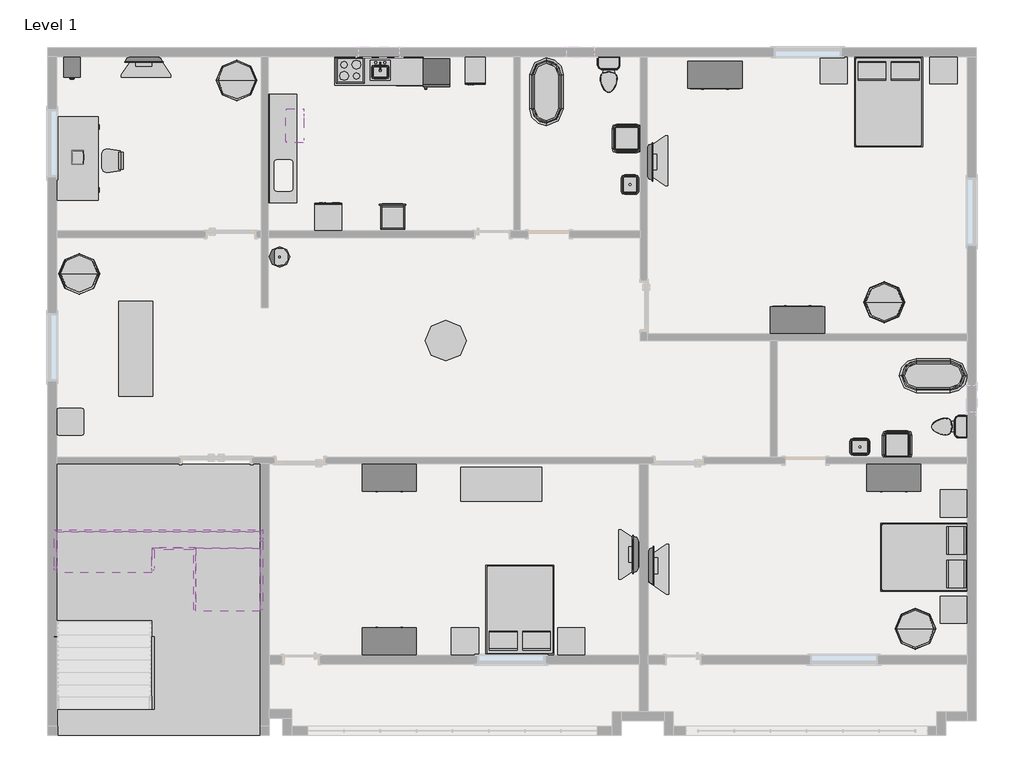
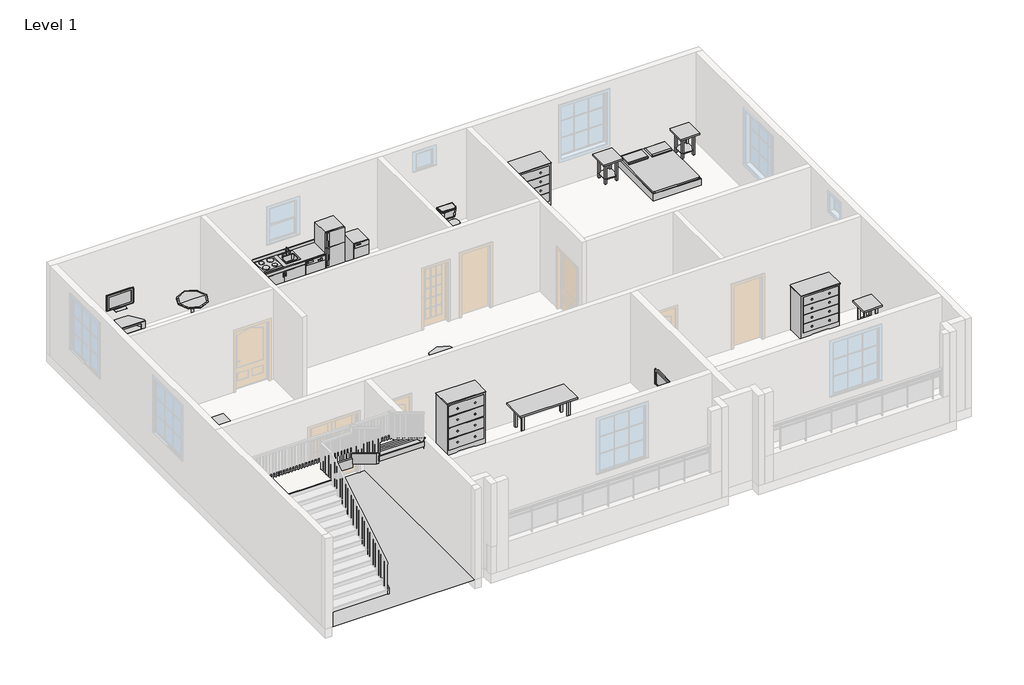
# One storey, part 4 of 4: 35 furniture elements, 10 proxies, 9 members, 8 flow terminals, 2 geographic elements, 1 slab, 1 stair flight.
"""IFC4 building model written with IfcOpenShell, lengths in millimetres."""

from ifc_helpers import new_model, si_unit, frame, origin, place, context, project, spatial, polyline, outline, extrude, faceted_brep, triangles, transform, mapped, element, save
from components import entourage_4c8cfd20, proxy_7e1014cc, proxy_a6faaae8, proxy_45b28599, kitchenette_medium_kitchenette_medium_844211aa, proxy_8a8d5ab2, proxy_8b8c2dc4, proxy_c523a7b7, flow_terminal_871c2e40, flow_terminal_d49f872f, flow_terminal_62a433f7, toilet_domestic_3d_toilet_domestic_3d_f7549cf7, toilet_domestic_3d_toilet_domestic_3d_183bbd19, flow_terminal_b374fae2, furniture_1d2926bd, furniture_d4d3357e, chair_desk_chair_desk_ccc35c8f, furniture_22cae41e, furniture_c6510c7c, furniture_2fc54265, furniture_2babcf72, furniture_9fa109b2, furniture_56245f3a, tv_stand_tv_stand_6ce107e5, furniture_92191dda, furniture_905aceb5, furniture_bcf351fa, furniture_5bc9ed15, furniture_a5b052b6, furniture_c80d6d9c, trash_can_trash_can_952d1acd, non_monolithic_landing_e2aaf49c, stair_flight_724757b1

model = new_model("IFC4")

# Units and contexts
model_context = context("Model", 3, world=origin())
ifc_project = project(units=[si_unit("LENGTHUNIT", "METRE", prefix="MILLI")], contexts=[model_context])

# Site, building, storey
site = spatial("IfcSite", under=ifc_project)
building = spatial("IfcBuilding", under=site)
storey = spatial("IfcBuildingStorey", under=building, Name="Level 1", Elevation=0.0)

# Proxies
placement = place(None, origin())
element("IfcBuildingElementProxy", 1, Name="Building Element Proxy", at=placement, inside=storey, context=model_context, shape_type="Tessellation", body=[
    triangles([(-19977.248053, 5318.025975, 0.0), (-15405.248053, 5318.025975, 0.0), (-15405.248053, -777.9740976, 0.0), (-19951.8472778, -777.9740976, 0.0)], [[1, 4, 2], [3, 2, 4]], closed=False),
])
entourage_shape = entourage_4c8cfd20(model_context)
element("IfcBuildingElementProxy", 2, Name="Entourage", at=placement, inside=storey, context=model_context, shape_type="MappedRepresentation", body=[
    mapped(entourage_shape, transform((-19545.4480019, 12201.4258877, 762.0), x_axis=(0.0, 1.0000000000000002, 0.0), y_axis=(-1.0000000000000002, 0.0, 0.0), z_axis=(0.0, 0.0, 1.0))),
])
proxy_shape = proxy_7e1014cc(model_context)
element("IfcBuildingElementProxy", 3, Name="18\" x 24\" x 34 1/2\"", ObjectType="18\" x 24\" x 34 1/2\"", at=placement, inside=storey, context=model_context, shape_type="MappedRepresentation", body=[
    mapped(proxy_shape, transform((-10885.3654704, 13890.776323, 0.0), x_axis=(1.0000000000000002, 0.0, 0.0), y_axis=(0.0, 1.0000000000000002, 0.0), z_axis=(0.0, 0.0, 1.0))),
])
proxy_2_shape = proxy_a6faaae8(model_context)
element("IfcBuildingElementProxy", 4, Name="Cook Top-4 Unit2 : 22\" x 20\"", ObjectType="Cook Top-4 Unit2 : 22\" x 20\"", at=placement, inside=storey, context=model_context, shape_type="MappedRepresentation", body=[
    mapped(proxy_2_shape, transform((-13385.9480019, 14157.2258877, 0.0), x_axis=(1.0, 0.0, 0.0), y_axis=(0.0, 1.0, 0.0), z_axis=(0.0, 0.0, 1.0))),
])
proxy_3_shape = proxy_45b28599(model_context)
element("IfcBuildingElementProxy", 5, Name="Dishwasher : 24\" x 24\" x 34\"", ObjectType="Dishwasher : 24\" x 24\" x 34\"", at=placement, inside=storey, context=model_context, shape_type="MappedRepresentation", body=[
    mapped(proxy_3_shape, transform((-13498.9305334, 11121.6754525, 0.0), x_axis=(-1.0000000000000004, 0.0, 0.0), y_axis=(0.0, -1.0000000000000004, 0.0), z_axis=(0.0, 0.0, 1.0))),
])
element("IfcBuildingElementProxy", 6, Name="Dishwasher : 24\" x 24\" x 34\"", ObjectType="Dishwasher : 24\" x 24\" x 34\"", at=placement, inside=storey, context=model_context, shape_type="MappedRepresentation", body=[
    mapped(proxy_3_shape, transform((-12434.7654704, 13865.376323, 0.0), x_axis=(1.0, 0.0, 0.0), y_axis=(0.0, 1.0, 0.0), z_axis=(0.0, 0.0, 1.0))),
])
kitchenette_medium_kitchenette_medium_shape = kitchenette_medium_kitchenette_medium_844211aa(model_context)
element("IfcBuildingElementProxy", 7, Name="Kitchenette - Medium : Kitchenette - Medium", ObjectType="Kitchenette - Medium : Kitchenette - Medium", at=placement, inside=storey, context=model_context, shape_type="MappedRepresentation", body=[
    mapped(kitchenette_medium_kitchenette_medium_shape, transform((-13061.7857068, 14462.0258877, 0.0), x_axis=(1.0, 0.0, 0.0), y_axis=(0.0, 1.0, 0.0), z_axis=(0.0, 0.0, 1.0))),
])
proxy_4_shape = proxy_8a8d5ab2(model_context)
element("IfcBuildingElementProxy", 8, Name="Microwave : 30\" x 16\" x 18\"", ObjectType="Microwave : 30\" x 16\" x 18\"", at=placement, inside=storey, context=model_context, shape_type="MappedRepresentation", body=[
    mapped(proxy_4_shape, transform((-14983.6285077, 12412.3330104, 304.8), x_axis=(0.0, 1.0000000000000004, 0.0), y_axis=(-1.0000000000000004, 0.0, 0.0), z_axis=(0.0, 0.0, 1.0))),
])
proxy_5_shape = proxy_8b8c2dc4(model_context)
element("IfcBuildingElementProxy", 9, Name="Oven Double-Built-in : 21 1/2\" x 39 1/4\" x 21\"", ObjectType="Oven Double-Built-in : 21 1/2\" x 39 1/4\" x 21\"", at=placement, inside=storey, context=model_context, shape_type="MappedRepresentation", body=[
    mapped(proxy_5_shape, transform((-12468.6229292, 10996.2917467, 0.0), x_axis=(-1.000000000000001, 0.0, 0.0), y_axis=(0.0, -1.000000000000001, 0.0), z_axis=(0.0, 0.0, 1.0))),
])
proxy_6_shape = proxy_c523a7b7(model_context)
element("IfcBuildingElementProxy", 10, Name="Refrigerator : 24\" x 25\" LH", ObjectType="Refrigerator : 24\" x 25\" LH", at=placement, inside=storey, context=model_context, shape_type="MappedRepresentation", body=[
    mapped(proxy_6_shape, transform((-11449.1980019, 14111.5769163, 0.0), x_axis=(1.0, 0.0, 0.0), y_axis=(0.0, 1.0, 0.0), z_axis=(0.0, 0.0, 1.0))),
])

# Flow terminals
flow_terminal_shape = flow_terminal_871c2e40(model_context)
element("IfcFlowTerminal", 11, ObjectType="Sink Kitchen-Island : 18\" x 18\"", at=placement, inside=storey, context=model_context, shape_type="MappedRepresentation", body=[
    mapped(flow_terminal_shape, transform((-12728.5372424, 14154.8804866, -14.4), x_axis=(1.0, 0.0, 0.0), y_axis=(0.0, 1.0, 0.0), z_axis=(0.0, 0.0, 1.0))),
])
flow_terminal_2_shape = flow_terminal_d49f872f(model_context)
element("IfcFlowTerminal", 12, ObjectType="Sink Vanity-Round : 19\" x 19\"", at=placement, inside=storey, context=model_context, shape_type="MappedRepresentation", body=[
    mapped(flow_terminal_2_shape, transform((-14887.9676231, 9869.5741472, 431.8), x_axis=(0.0, 1.0000000000000002, 0.0), y_axis=(-1.0000000000000002, 0.0, 0.0), z_axis=(0.0, 0.0, 1.0))),
])
flow_terminal_3_shape = flow_terminal_62a433f7(model_context)
element("IfcFlowTerminal", 13, ObjectType="Sink Vanity-Square : 20\" x 18\"", at=placement, inside=storey, context=model_context, shape_type="MappedRepresentation", body=[
    mapped(flow_terminal_3_shape, transform((-1927.5587613, 5650.5712889, 609.6), x_axis=(-1.0000000000000004, 0.0, 0.0), y_axis=(0.0, -1.0000000000000004, 0.0), z_axis=(0.0, 0.0, 1.0))),
])
element("IfcFlowTerminal", 14, ObjectType="Sink Vanity-Square : 20\" x 18\"", at=placement, inside=storey, context=model_context, shape_type="MappedRepresentation", body=[
    mapped(flow_terminal_3_shape, transform((-7050.993403, 11607.5151283, 609.6), x_axis=(0.0, -1.0000000000000004, 0.0), y_axis=(1.0000000000000004, 0.0, 0.0), z_axis=(0.0, 0.0, 1.0))),
])
toilet_domestic_3d_toilet_domestic_3d_shape = toilet_domestic_3d_toilet_domestic_3d_f7549cf7(model_context)
toilet_domestic_3d_toilet_domestic_3d_2_shape = toilet_domestic_3d_toilet_domestic_3d_183bbd19(model_context)
element("IfcFlowTerminal", 15, ObjectType="Toilet-Domestic-3D : Toilet-Domestic-3D", at=placement, inside=storey, context=model_context, shape_type="MappedRepresentation", body=[
    mapped(toilet_domestic_3d_toilet_domestic_3d_shape, transform((-24.9440292, 6156.2258877, 0.0), x_axis=(0.0, -1.0000000000000004, 0.0), y_axis=(1.0000000000000004, 0.0, 0.0), z_axis=(0.0, 0.0, 1.0))),
    mapped(toilet_domestic_3d_toilet_domestic_3d_2_shape, transform((-24.9440292, 6156.2258877, 0.0), x_axis=(0.0, -1.0000000000000004, 0.0), y_axis=(1.0000000000000004, 0.0, 0.0), z_axis=(0.0, 0.0, 1.0))),
])
element("IfcFlowTerminal", 16, ObjectType="Toilet-Domestic-3D : Toilet-Domestic-3D", at=placement, inside=storey, context=model_context, shape_type="MappedRepresentation", body=[
    mapped(toilet_domestic_3d_toilet_domestic_3d_shape, transform((-7582.0480019, 13967.3298604, 0.0), x_axis=(1.0, 0.0, 0.0), y_axis=(0.0, 1.0, 0.0), z_axis=(0.0, 0.0, 1.0))),
    mapped(toilet_domestic_3d_toilet_domestic_3d_2_shape, transform((-7582.0480019, 13967.3298604, 0.0), x_axis=(1.0, 0.0, 0.0), y_axis=(0.0, 1.0, 0.0), z_axis=(0.0, 0.0, 1.0))),
])
flow_terminal_4_shape = flow_terminal_b374fae2(model_context)
element("IfcFlowTerminal", 17, ObjectType="Tub-Free Standing-3D : 30\" x 60\"", at=placement, inside=storey, context=model_context, shape_type="MappedRepresentation", body=[
    mapped(flow_terminal_4_shape, transform((-292.2480019, 7299.2258877, 0.0), x_axis=(0.0, -1.0000000000000004, 0.0), y_axis=(1.0000000000000004, 0.0, 0.0), z_axis=(0.0, 0.0, 1.0))),
])
element("IfcFlowTerminal", 18, ObjectType="Tub-Free Standing-3D : 30\" x 60\"", at=placement, inside=storey, context=model_context, shape_type="MappedRepresentation", body=[
    mapped(flow_terminal_4_shape, transform((-8979.0480019, 13674.6258877, 0.0), x_axis=(1.0, 0.0, 0.0), y_axis=(0.0, 1.0, 0.0), z_axis=(0.0, 0.0, 1.0))),
])

# Furniture
furniture_shape = furniture_1d2926bd(model_context)
element("IfcFurniture", 19, ObjectType="Bed-Box : Queen 60\" x 79\"", at=placement, inside=storey, context=model_context, shape_type="MappedRepresentation", body=[
    mapped(furniture_shape, transform((-235.6184937, 3561.6783468, 0.0), x_axis=(0.0, -1.0, 0.0), y_axis=(1.0, 0.0, 0.0), z_axis=(0.0, 0.0, 1.0))),
])
element("IfcFurniture", 20, ObjectType="Bed-Box : Queen 60\" x 79\"", at=placement, inside=storey, context=model_context, shape_type="MappedRepresentation", body=[
    mapped(furniture_shape, transform((-9236.7955428, 1806.9963796, 0.0), x_axis=(-0.9999999999999998, 0.0, 0.0), y_axis=(0.0, -0.9999999999999998, 0.0), z_axis=(0.0, 0.0, 1.0))),
])
element("IfcFurniture", 21, ObjectType="Bed-Box : Queen 60\" x 79\"", at=placement, inside=storey, context=model_context, shape_type="MappedRepresentation", body=[
    mapped(furniture_shape, transform((-1634.7004609, 13680.4553959, 0.0), x_axis=(1.000000000000001, 0.0, 0.0), y_axis=(0.0, 1.000000000000001, 0.0), z_axis=(0.0, 0.0, 1.0))),
])
furniture_2_shape = furniture_d4d3357e(model_context)
element("IfcFurniture", 22, ObjectType="Cabinet-File 5 Drawer : 15\" x 18\"", at=placement, inside=storey, context=model_context, shape_type="MappedRepresentation", body=[
    mapped(furniture_2_shape, transform((-19506.4515548, 14375.5601879, 0.0), x_axis=(1.0, 0.0, 0.0), y_axis=(0.0, 1.0, 0.0), z_axis=(0.0, 0.0, 1.0))),
])
chair_desk_chair_desk_shape = chair_desk_chair_desk_ccc35c8f(model_context)
element("IfcFurniture", 23, ObjectType="Chair-Desk : Chair-Desk", at=placement, inside=storey, context=model_context, shape_type="MappedRepresentation", body=[
    mapped(chair_desk_chair_desk_shape, transform((-18554.8480019, 12125.2258877, 0.0), x_axis=(0.0, 1.0000000000000002, 0.0), y_axis=(-1.0000000000000002, 0.0, 0.0), z_axis=(0.0, 0.0, 1.0))),
])
furniture_3_shape = furniture_22cae41e(model_context)
element("IfcFurniture", 24, ObjectType="Counter Top w Sink Hole : 24\" Depth", at=placement, inside=storey, context=model_context, shape_type="MappedRepresentation", body=[
    mapped(furniture_3_shape, transform((-15227.4480019, 12385.8881828, 0.0), x_axis=(0.0, 1.0000000000000009, 0.0), y_axis=(-1.0000000000000009, 0.0, 0.0), z_axis=(0.0, 0.0, 1.0))),
])
furniture_4_shape = furniture_c6510c7c(model_context)
element("IfcFurniture", 25, ObjectType="Counter Top w Sink Hole : 24\" Depth", at=placement, inside=storey, context=model_context, shape_type="MappedRepresentation", body=[
    mapped(furniture_4_shape, transform((-12528.3857068, 14462.0258877, -14.4), x_axis=(1.0, 0.0, 0.0), y_axis=(0.0, 1.0, 0.0), z_axis=(0.0, 0.0, 1.0))),
])
furniture_5_shape = furniture_2fc54265(model_context)
element("IfcFurniture", 26, ObjectType="Desk : 72\" x 36\"", at=placement, inside=storey, context=model_context, shape_type="MappedRepresentation", body=[
    mapped(furniture_5_shape, transform((-19977.2480019, 13090.4258877, 0.0), x_axis=(0.0, -1.0000000000000007, 0.0), y_axis=(1.0000000000000007, 0.0, 0.0), z_axis=(0.0, 0.0, 1.0))),
])
furniture_6_shape = furniture_2babcf72(model_context)
element("IfcFurniture", 27, ObjectType="Dresser : 48\" x 60\" x 24\"", at=placement, inside=storey, context=model_context, shape_type="MappedRepresentation", body=[
    mapped(furniture_6_shape, transform((-912.054742, 5376.3888418, 0.0), x_axis=(1.0, 0.0, 0.0), y_axis=(0.0, 1.0, 0.0), z_axis=(0.0, 0.0, 1.0))),
])
element("IfcFurniture", 28, ObjectType="Dresser : 48\" x 60\" x 24\"", at=placement, inside=storey, context=model_context, shape_type="MappedRepresentation", body=[
    mapped(furniture_6_shape, transform((-3609.4412617, 8180.6629336, 0.0), x_axis=(-1.0000000000000004, 0.0, 0.0), y_axis=(0.0, -1.0000000000000004, 0.0), z_axis=(0.0, 0.0, 1.0))),
])
element("IfcFurniture", 29, ObjectType="Dresser : 48\" x 60\" x 24\"", at=placement, inside=storey, context=model_context, shape_type="MappedRepresentation", body=[
    mapped(furniture_6_shape, transform((-4925.254742, 14418.7888418, 0.0), x_axis=(1.0000000000000007, 0.0, 0.0), y_axis=(0.0, 1.0000000000000007, 0.0), z_axis=(0.0, 0.0, 1.0))),
])
furniture_7_shape = furniture_9fa109b2(model_context)
element("IfcFurniture", 30, ObjectType="Dresser : 48\" x 72\" x 24\"", at=placement, inside=storey, context=model_context, shape_type="MappedRepresentation", body=[
    mapped(furniture_7_shape, transform((-12778.8412617, 967.0629336, 0.0), x_axis=(-1.0000000000000004, 0.0, 0.0), y_axis=(0.0, -1.0000000000000004, 0.0), z_axis=(0.0, 0.0, 1.0))),
])
element("IfcFurniture", 31, ObjectType="Dresser : 48\" x 72\" x 24\"", at=placement, inside=storey, context=model_context, shape_type="MappedRepresentation", body=[
    mapped(furniture_7_shape, transform((-12240.454742, 5376.3888418, 0.0), x_axis=(1.0, 0.0, 0.0), y_axis=(0.0, 1.0, 0.0), z_axis=(0.0, 0.0, 1.0))),
])
furniture_8_shape = furniture_56245f3a(model_context)
element("IfcFurniture", 32, ObjectType="TV - Flat Screen : 32\"", at=placement, inside=storey, context=model_context, shape_type="MappedRepresentation", body=[
    mapped(furniture_8_shape, transform((-6979.8708936, 3282.0813736, 914.4), x_axis=(0.0, -1.0000000000000004, 0.0), y_axis=(1.0000000000000004, 0.0, 0.0), z_axis=(0.0, 0.0, 1.0))),
])
element("IfcFurniture", 33, ObjectType="TV - Flat Screen : 32\"", at=placement, inside=storey, context=model_context, shape_type="MappedRepresentation", body=[
    mapped(furniture_8_shape, transform((-6634.5093782, 3035.9704019, 914.4), x_axis=(0.0, 1.0, 0.0), y_axis=(-1.0, 0.0, 0.0), z_axis=(0.0, 0.0, 1.0))),
])
element("IfcFurniture", 34, ObjectType="TV - Flat Screen : 32\"", at=placement, inside=storey, context=model_context, shape_type="MappedRepresentation", body=[
    mapped(furniture_8_shape, transform((-6659.9093782, 12103.7704019, 914.4), x_axis=(0.0, 1.0000000000000002, 0.0), y_axis=(-1.0000000000000002, 0.0, 0.0), z_axis=(0.0, 0.0, 1.0))),
])
element("IfcFurniture", 35, ObjectType="TV - Flat Screen : 32\"", at=placement, inside=storey, context=model_context, shape_type="MappedRepresentation", body=[
    mapped(furniture_8_shape, transform((-18017.5034877, 14403.4872641, 914.4), x_axis=(1.0, 0.0, 0.0), y_axis=(0.0, 1.0, 0.0), z_axis=(0.0, 0.0, 1.0))),
])
tv_stand_tv_stand_shape = tv_stand_tv_stand_6ce107e5(model_context)
element("IfcFurniture", 36, ObjectType="TV Stand : TV Stand", at=placement, inside=storey, context=model_context, shape_type="MappedRepresentation", body=[
    mapped(tv_stand_tv_stand_shape, transform((-6896.2480019, 3411.2138898, 0.0), x_axis=(0.0, -1.0, 0.0), y_axis=(1.0, 0.0, 0.0), z_axis=(0.0, 0.0, 1.0))),
])
element("IfcFurniture", 37, ObjectType="TV Stand : TV Stand", at=placement, inside=storey, context=model_context, shape_type="MappedRepresentation", body=[
    mapped(tv_stand_tv_stand_shape, transform((-6693.0480019, 2830.6378857, 0.0), x_axis=(0.0, 1.0000000000000002, 0.0), y_axis=(-1.0000000000000002, 0.0, 0.0), z_axis=(0.0, 0.0, 1.0))),
])
element("IfcFurniture", 38, ObjectType="TV Stand : TV Stand", at=placement, inside=storey, context=model_context, shape_type="MappedRepresentation", body=[
    mapped(tv_stand_tv_stand_shape, transform((-6718.4480019, 12000.0378857, 0.0), x_axis=(0.0, 1.0000000000000002, 0.0), y_axis=(-1.0000000000000002, 0.0, 0.0), z_axis=(0.0, 0.0, 1.0))),
])
element("IfcFurniture", 39, ObjectType="TV Stand : TV Stand", at=placement, inside=storey, context=model_context, shape_type="MappedRepresentation", body=[
    mapped(tv_stand_tv_stand_shape, transform((-18095.8360039, 14462.0258877, 0.0), x_axis=(1.0, 0.0, 0.0), y_axis=(0.0, 1.0, 0.0), z_axis=(0.0, 0.0, 1.0))),
])
furniture_9_shape = furniture_92191dda(model_context)
element("IfcFurniture", 40, ObjectType="Table-Dining : 30\" x 84\" x 22\"", at=placement, inside=storey, context=model_context, shape_type="MappedRepresentation", body=[
    mapped(furniture_9_shape, transform((-18104.0369241, 7890.5601211, 0.0), x_axis=(0.0, 1.0, 0.0), y_axis=(-1.0, 0.0, 0.0), z_axis=(0.0, 0.0, 1.0))),
])
furniture_10_shape = furniture_905aceb5(model_context)
element("IfcFurniture", 41, ObjectType="Table-Dining Round w Chairs : 36\" Diameter", at=placement, inside=storey, context=model_context, shape_type="MappedRepresentation", body=[
    mapped(furniture_10_shape, transform((-11343.3299691, 8271.5045763, 0.0), x_axis=(1.0, 0.0, 0.0), y_axis=(0.0, 1.0, 0.0), z_axis=(0.0, 0.0, 1.0))),
])
furniture_11_shape = furniture_bcf351fa(model_context)
element("IfcFurniture", 42, ObjectType="Table-End : 24\" x 24\"", at=placement, inside=storey, context=model_context, shape_type="MappedRepresentation", body=[
    mapped(furniture_11_shape, transform((-19980.9816322, 6111.7758877, 0.0), x_axis=(1.0, 0.0, 0.0), y_axis=(0.0, 1.0, 0.0), z_axis=(0.0, 0.0, 1.0))),
])
furniture_12_shape = furniture_5bc9ed15(model_context)
element("IfcFurniture", 43, ObjectType="Table-Night Stand : 24\" x 24\" x 30\"", at=placement, inside=storey, context=model_context, shape_type="MappedRepresentation", body=[
    mapped(furniture_12_shape, transform((-143.5816322, 4124.2258877, 0.0), x_axis=(1.0, 0.0, 0.0), y_axis=(0.0, 1.0, 0.0), z_axis=(0.0, 0.0, 1.0))),
])
element("IfcFurniture", 44, ObjectType="Table-Night Stand : 24\" x 24\" x 30\"", at=placement, inside=storey, context=model_context, shape_type="MappedRepresentation", body=[
    mapped(furniture_12_shape, transform((-143.5816322, 1736.6258877, 0.0), x_axis=(1.0, 0.0, 0.0), y_axis=(0.0, 1.0, 0.0), z_axis=(0.0, 0.0, 1.0))),
])
element("IfcFurniture", 45, ObjectType="Table-Night Stand : 24\" x 24\" x 30\"", at=placement, inside=storey, context=model_context, shape_type="MappedRepresentation", body=[
    mapped(furniture_12_shape, transform((-372.1816322, 13852.4258877, 0.0), x_axis=(1.0, 0.0, 0.0), y_axis=(0.0, 1.0, 0.0), z_axis=(0.0, 0.0, 1.0))),
])
element("IfcFurniture", 46, ObjectType="Table-Night Stand : 24\" x 24\" x 30\"", at=placement, inside=storey, context=model_context, shape_type="MappedRepresentation", body=[
    mapped(furniture_12_shape, transform((-2835.9816322, 13852.4258877, 0.0), x_axis=(1.0, 0.0, 0.0), y_axis=(0.0, 1.0, 0.0), z_axis=(0.0, 0.0, 1.0))),
])
element("IfcFurniture", 47, ObjectType="Table-Night Stand : 24\" x 24\" x 30\"", at=placement, inside=storey, context=model_context, shape_type="MappedRepresentation", body=[
    mapped(furniture_12_shape, transform((-8728.7816322, 1025.4258877, 0.0), x_axis=(1.0, 0.0, 0.0), y_axis=(0.0, 1.0, 0.0), z_axis=(0.0, 0.0, 1.0))),
])
element("IfcFurniture", 48, ObjectType="Table-Night Stand : 24\" x 24\" x 30\"", at=placement, inside=storey, context=model_context, shape_type="MappedRepresentation", body=[
    mapped(furniture_12_shape, transform((-11116.3816322, 1025.4258877, 0.0), x_axis=(1.0, 0.0, 0.0), y_axis=(0.0, 1.0, 0.0), z_axis=(0.0, 0.0, 1.0))),
])
furniture_13_shape = furniture_a5b052b6(model_context)
element("IfcFurniture", 49, ObjectType="Table-Rectangular : 72\" x 30\"", at=placement, inside=storey, context=model_context, shape_type="MappedRepresentation", body=[
    mapped(furniture_13_shape, transform((-9995.0480019, 4860.8258877, 0.0), x_axis=(1.0, 0.0, 0.0), y_axis=(0.0, 1.0, 0.0), z_axis=(0.0, 0.0, 1.0))),
])
furniture_14_shape = furniture_c80d6d9c(model_context)
element("IfcFurniture", 50, ObjectType="Table-Round : 36\" Diameter", at=placement, inside=storey, context=model_context, shape_type="MappedRepresentation", body=[
    mapped(furniture_14_shape, transform((-15938.6480019, 13928.6258877, 0.0), x_axis=(1.0, 0.0, 0.0), y_axis=(0.0, 1.0, 0.0), z_axis=(0.0, 0.0, 1.0))),
])
element("IfcFurniture", 51, ObjectType="Table-Round : 36\" Diameter", at=placement, inside=storey, context=model_context, shape_type="MappedRepresentation", body=[
    mapped(furniture_14_shape, transform((-19469.2480019, 9585.2258877, 0.0), x_axis=(1.0, 0.0, 0.0), y_axis=(0.0, 1.0, 0.0), z_axis=(0.0, 0.0, 1.0))),
])
element("IfcFurniture", 52, ObjectType="Table-Round : 36\" Diameter", at=placement, inside=storey, context=model_context, shape_type="MappedRepresentation", body=[
    mapped(furniture_14_shape, transform((-694.4469099, 1615.7956449, 0.0), x_axis=(1.0, 0.0, 0.0), y_axis=(0.0, 1.0, 0.0), z_axis=(0.0, 0.0, 1.0))),
])
element("IfcFurniture", 53, ObjectType="Table-Round : 36\" Diameter", at=placement, inside=storey, context=model_context, shape_type="MappedRepresentation", body=[
    mapped(furniture_14_shape, transform((-1395.5576114, 8948.7567865, 0.0), x_axis=(1.0, 0.0, 0.0), y_axis=(0.0, 1.0, 0.0), z_axis=(0.0, 0.0, 1.0))),
])

# Geographic elements
trash_can_trash_can_shape = trash_can_trash_can_952d1acd(model_context)
element("IfcGeographicElement", 54, ObjectType="Trash Can : Trash Can", at=placement, inside=storey, context=model_context, shape_type="MappedRepresentation", body=[
    mapped(trash_can_trash_can_shape, transform((-1105.0480019, 5749.8258877, 0.0), x_axis=(1.0, 0.0, 0.0), y_axis=(0.0, 1.0, 0.0), z_axis=(0.0, 0.0, 1.0))),
])
element("IfcGeographicElement", 55, ObjectType="Trash Can : Trash Can", at=placement, inside=storey, context=model_context, shape_type="MappedRepresentation", body=[
    mapped(trash_can_trash_can_shape, transform((-7175.6480019, 12633.2258877, 0.0), x_axis=(1.0, 0.0, 0.0), y_axis=(0.0, 1.0, 0.0), z_axis=(0.0, 0.0, 1.0))),
])

# Members
element("IfcMember", 56, ObjectType="Stringer - 2\" Width", at=placement, inside=storey, context=model_context, shape_type="SweptSolid", body=[
    extrude(outline(polyline([(-193.7741123, 0.0), (-193.7741123, 212.114512), (2934.766943, 2108.2), (3019.9213995, 1803.4), (44.3113995, 0.0), (-193.7741123, 0.0)])), frame((-20028.0480019, 0.0, 0.0), z_axis=(1.0, 0.0, 0.0), x_axis=(0.0, 1.0, 0.0)), (0.0, 0.0, 1.0), 50.8),
])
element("IfcMember", 57, ObjectType="Stringer - 2\" Width", at=placement, inside=storey, context=model_context, shape_type="SweptSolid", body=[
    extrude(outline(polyline([(-193.7741123, 0.0), (-193.7741123, 212.114512), (2934.766943, 2108.2), (3019.9213995, 1803.4), (44.3113995, 0.0), (-193.7741123, 0.0)])), frame((-17843.6480019, 0.0, 0.0), z_axis=(1.0, 0.0, 0.0), x_axis=(0.0, 1.0, 0.0)), (0.0, 0.0, 1.0), 50.8),
])
element("IfcMember", 58, ObjectType="Stringer - 2\" Width", at=placement, inside=storey, context=model_context, shape_type="SweptSolid", body=[
    extrude(outline(polyline([(3662.6848325, 2108.2), (3577.530376, 1803.4), (2041.4258877, 2734.3724171), (2041.4258877, 3090.7811786), (3662.6848325, 2108.2)])), frame((-15405.2480019, 0.0, 0.0), z_axis=(1.0, 0.0, 0.0), x_axis=(0.0, 1.0, 0.0)), (0.0, 0.0, 1.0), 50.8),
])
element("IfcMember", 59, ObjectType="Stringer - 2\" Width", at=placement, inside=storey, context=model_context, shape_type="SweptSolid", body=[
    extrude(outline(polyline([(3438.4258877, 2244.114512), (3438.4258877, 1887.7057504), (2041.4258877, 2734.3724171), (2041.4258877, 3090.7811786), (3438.4258877, 2244.114512)])), frame((-16903.8480019, 0.0, 0.0), z_axis=(1.0, 0.0, 0.0), x_axis=(0.0, 1.0, 0.0)), (0.0, 0.0, 1.0), 50.8),
])
element("IfcMember", 60, ObjectType="Stringer - 2\" Width", at=placement, inside=storey, context=model_context, shape_type="Brep", body=[
    faceted_brep([(-15405.2480019, 3662.6848325, 2108.2), (-15354.4480019, 3662.6848325, 2108.2), (-15354.4480019, 3844.8258877, 2108.2), (-15405.2480019, 3794.0258877, 2108.2), (-15405.2480019, 3577.530376, 1803.4), (-15405.2480019, 3794.0258877, 1803.4), (-15354.4480019, 3577.530376, 1803.4), (-15354.4480019, 3844.8258877, 1803.4)], [[[0, 1, 2, 3]], [[4, 0, 3, 5]], [[6, 4, 5, 7]], [[1, 6, 7, 2]], [[1, 0, 4, 6]], [[2, 7, 5, 3]]]),
])
element("IfcMember", 61, ObjectType="Stringer - 2\" Width", at=placement, inside=storey, context=model_context, shape_type="SweptSolid", body=[
    extrude(outline(polyline([(-15354.4480019, 3844.8258877), (-15405.2480019, 3794.0258877), (-19977.2480019, 3794.0258877), (-20028.0480019, 3844.8258877), (-15354.4480019, 3844.8258877)])), frame((0.0, 0.0, 1803.4), z_axis=(0.0, 0.0, 1.0), x_axis=(1.0, 0.0, 0.0)), (0.0, 0.0, 1.0), 304.8),
])
element("IfcMember", 62, ObjectType="Stringer - 2\" Width", at=placement, inside=storey, context=model_context, shape_type="Brep", body=[
    faceted_brep([(-19977.2480019, 3794.0258877, 2108.2), (-20028.0480019, 3844.8258877, 2108.2), (-20028.0480019, 2934.766943, 2108.2), (-19977.2480019, 2934.766943, 2108.2), (-19977.2480019, 3794.0258877, 1803.4), (-19977.2480019, 3019.9213995, 1803.4), (-20028.0480019, 3844.8258877, 1803.4), (-20028.0480019, 3019.9213995, 1803.4)], [[[0, 1, 2, 3]], [[4, 0, 3, 5]], [[6, 4, 5, 7]], [[1, 6, 7, 2]], [[1, 0, 4, 6]], [[2, 7, 5, 3]]]),
])
element("IfcMember", 63, ObjectType="Stringer - 2\" Width", at=placement, inside=storey, context=model_context, shape_type="Brep", body=[
    faceted_brep([(-17843.6480019, 2934.766943, 2108.2), (-17792.8480019, 2934.766943, 2108.2), (-17792.8480019, 3387.6258877, 2108.2), (-17843.6480019, 3438.4258877, 2108.2), (-17843.6480019, 3019.9213995, 1803.4), (-17843.6480019, 3438.4258877, 1803.4), (-17792.8480019, 3019.9213995, 1803.4), (-17792.8480019, 3387.6258877, 1803.4)], [[[0, 1, 2, 3]], [[4, 0, 3, 5]], [[6, 4, 5, 7]], [[1, 6, 7, 2]], [[1, 0, 4, 6]], [[2, 7, 5, 3]]]),
])
element("IfcMember", 64, ObjectType="Stringer - 2\" Width", at=placement, inside=storey, context=model_context, shape_type="SweptSolid", body=[
    extrude(outline(polyline([(-17792.8480019, 3387.6258877), (-17843.6480019, 3438.4258877), (-16903.8480019, 3438.4258877), (-16903.8480019, 3387.6258877), (-17792.8480019, 3387.6258877)])), frame((0.0, 0.0, 1803.4), z_axis=(0.0, 0.0, 1.0), x_axis=(1.0, 0.0, 0.0)), (0.0, 0.0, 1.0), 304.8),
])

# Slab
non_monolithic_landing_shape = non_monolithic_landing_e2aaf49c(model_context)
element("IfcSlab", 65, ObjectType="Non-Monolithic Landing", at=placement, inside=storey, context=model_context, shape_type="MappedRepresentation", body=[
    mapped(non_monolithic_landing_shape, transform((0.0, 0.0, 0.0), x_axis=(1.0, 0.0, 0.0), y_axis=(0.0, 1.0, 0.0), z_axis=(0.0, 0.0, 1.0))),
])

# Stair flight
stair_flight_shape = stair_flight_724757b1(model_context)
element("IfcStairFlight", 66, ObjectType="2\" Tread 1\" Nosing 1/4\" Riser", at=placement, inside=storey, context=model_context, shape_type="MappedRepresentation", body=[
    mapped(stair_flight_shape, transform((0.0, 0.0, 0.0), x_axis=(1.0, 0.0, 0.0), y_axis=(0.0, 1.0, 0.0), z_axis=(0.0, 0.0, 1.0))),
])

save(model, "model.ifc")

# Revit data of these elements
# Type
#   built-in parameter 1005195 = "RPC-16-N04H-AQSP-D1N4-43SU-6GKQ-C3KU-1C"
#   Height = 0
# Type "18\" x 24\" x 34 1/2\""
#   Label = "T"
#   Assembly Code = "E1090400"
#   Depth = 2' - 0"
#   Height = 2' - 10 1/2"
#   Width = 1' - 6"
#   Panel Face Material = Plastic, Opaque Black
#   Trach Compact. Material = Steel, Paint Finish, Ivory, Matte
#   Default Elevation = 0
# Type "Cook Top-4 Unit2 : 22\" x 20\""
#   Depth = 1' - 8"
#   Width = 1' - 10"
#   Burner Material = Steel, Chrome Plated
#   Cooktop Material = Steel, Polished
#   Default Elevation = 0
#   Assembly Code = ""
# Type "Dishwasher : 24\" x 24\" x 34\""
#   Label = "DW"
#   Assembly Code = "E1090400"
#   Depth = 2' - 0"
#   Height = 2' - 10"
#   Width = 2' - 0"
#   Dishwasher Material = Steel, Paint Finish, Ivory, Glossy
#   Panel Face Material = Plastic, Opaque Black
#   Default Elevation = 0
# Type "Kitchenette - Medium : Kitchenette - Medium"
#   Assembly Code = "E1090400"
#   Counter Length = 6' - 6"
#   Cabinet Width = 4' - 6"
#   Cabinet Height = 2' - 10 1/2"
#   Cabinet Depth = 2' - 0"
#   Toe Depth = 0' - 3"
#   Toe Height = 0' - 3 1/2"
#   Cabinet Material = Cabinets
#   Door/Drawer Material = Cabinets
#   Handle Material = Cabinets - Handles
#   Default Elevation = 0
# Type "Microwave : 30\" x 16\" x 18\""
#   Assembly Code = "E1090400"
#   Depth = 1' - 4"
#   Height = 1' - 6"
#   Width = 2' - 6"
#   Microwave Material = Laminate, Ivory, Matte
#   Default Elevation = 0
# Type "Oven Double-Built-in : 21 1/2\" x 39 1/4\" x 21\""
#   Label = "OVEN"
#   Assembly Code = "E1090400"
#   Depth = 1' - 9"
#   Height = 3' - 3 1/4"
#   Width = 1' - 9 1/2"
#   Oven Material = Metal - Stainless Steel, Polished
#   Default Elevation = 0
# Type "Refrigerator : 24\" x 25\" LH"
#   Label = "REF."
#   Assembly Code = "E1090400"
#   Depth = 2' - 0 3/4"
#   Handle = 0' - 1 1/2"
#   Height = 5' - 3 1/2"
#   Rear Clearance = 0' - 2"
#   Top Door Height = 1' - 8"
#   Width = 1' - 11 1/2"
#   Material = Steel, Paint Finish, Ivory, Glossy
#   Default Elevation = 0
# Type "Sink Kitchen-Island : 18\" x 18\""
#   Assembly Code = "D2010410"
#   Counter Height = 3' - 0"
#   Depth = 1' - 6"
#   Width = 1' - 6"
#   Faucet Material = Steel, Polished
#   Sink Material = Steel, Polished
#   Default Elevation = 0
# Type "Sink Vanity-Round : 19\" x 19\""
#   Assembly Code = "D2010400"
#   Top Of Counter = 2' - 7"
#   Basin Material = Porcelain, Linen
#   Faucet Material = Steel, Polished
#   Default Elevation = 0
# Type "Sink Vanity-Square : 20\" x 18\""
#   Assembly Code = "D2010400"
#   Counter Height = 2' - 7"
#   Depth = 1' - 6"
#   Width = 1' - 8"
#   Basin Material = Porcelain, Linen
#   Faucet Material = Steel, Polished
#   Default Elevation = 0
# Type "Toilet-Domestic-3D : Toilet-Domestic-3D"
#   Assembly Code = "D2010110"
#   Toilet - Bowl/Basin Material = Porcelain, Linen
#   Toilet - Seat Material = Laminate, Linen, Matte
#   Default Elevation = 0
# Type "Tub-Free Standing-3D : 30\" x 60\""
#   Assembly Code = "D2010110"
#   Height = 1' - 6"
#   Length = 5' - 0"
#   Width = 2' - 6"
#   Tub Material = Porcelain, Ivory
#   Default Elevation = 0
# Type "Bed-Box : Queen 60\" x 79\""
#   Assembly Code = "E2020200"
#   Length = 6' - 7"
#   Width = 5' - 0"
#   Frame Material = Birch
#   Mattress Material = Linen, White
#   Default Elevation = 0
# Type "Cabinet-File 5 Drawer : 15\" x 18\""
#   Assembly Code = "E2020200"
#   Depth = 1' - 6"
#   Height = 5' - 0"
#   Width = 1' - 3"
#   Cabinet Material = Steel, Paint Finish, Ivory, Glossy
#   Handle Material = Steel, Chrome Plated
#   Default Elevation = 0
# Type "Chair-Desk : Chair-Desk"
#   Assembly Code = "E2020200"
#   Seat/Back Material = Textile - Slate Blue
#   Base Material = Steel, Chrome Plated
#   Default Elevation = 0
# Type "Counter Top w Sink Hole : 24\" Depth"
#   Assembly Code = "C1030400"
#   Counter Thickness = 0' - 1 1/2"
#   Depth = 2' - 1"
#   Height = 3' - 0"
#   Length [instance default] = 8' - 0"
#   Sink Location [instance default] = 2' - 0"
#   Sink Location To Wall [instance default] = 0' - 6"
#   Sink Opening Depth [instance default] = 1' - 3"
#   Sink Opening Width [instance default] = 2' - 3"
#   Counter Top Material = none
#   Default Elevation = 0
# Type "Desk : 72\" x 36\""
#   Assembly Code = "E2020200"
#   Depth = 3' - 0"
#   Height = 2' - 6"
#   Leg Height = 0' - 6"
#   Width = 6' - 0"
#   Body Material = Laminate, Ivory, Matte
#   Handle/Leg Material = Steel, Chrome Plated
#   Top Material = Cherry
#   Default Elevation = 0
# Type "Dresser : 48\" x 60\" x 24\""
#   Assembly Code = "E2020200"
#   Depth = 2' - 0"
#   Height = 5' - 0"
#   Width = 4' - 0"
#   Dresser Material = Laminate - Ivory, Glossy
#   Drawer Material = Laminate, Ivory, Matte
#   Knob Material = Cherry
#   Default Elevation = 0
# Type "Dresser : 48\" x 72\" x 24\""
#   Assembly Code = "E2020200"
#   Depth = 2' - 0"
#   Height = 6' - 0"
#   Width = 4' - 0"
#   Dresser Material = Laminate - Ivory, Glossy
#   Drawer Material = Laminate, Ivory, Matte
#   Knob Material = Cherry
#   Default Elevation = 0
# Type "TV - Flat Screen : 32\""
#   SinAng = 0' - 0.0193"
#   L = 2' - 3.79372"
#   H = 1' - 3.6354"
#   Thickness = 0' - 4.33071"
#   Diagonal = 2' - 7.88976"
#   CosAng = 0' - 0.03431"
#   Stand [instance default] = yes
#   Default Elevation = 0
# Type "TV Stand : TV Stand"
#   Depth = 1' - 6"
#   Width = 3' - 8"
#   Height = 1' - 7 1/2"
#   Finish = Melamine - Gray
#   Default Elevation = 0
# Type "Table-Dining : 30\" x 84\" x 22\""
#   Assembly Code = "E2020200"
#   Height = 1' - 10"
#   Length = 7' - 0"
#   Width = 2' - 6"
#   Base Material = Steel, Chrome Plated
#   Top Material = Glass - Clear, Grey
#   Default Elevation = 0
# Type "Table-Dining Round w Chairs : 36\" Diameter"
#   Assembly Code = "E2020200"
#   Radius = 1' - 6"
#   Diameter = 3' - 0"
#   Height = 2' - 6"
#   Chairs = 4
#   Base Material = Pine
#   Top Material = Laminate, Linen, Matte
#   Default Elevation = 0
# Type "Table-End : 24\" x 24\""
#   Assembly Code = "E2020200"
#   Height = 2' - 6"
#   Length = 2' - 0"
#   Width = 2' - 0"
#   Base Material = Birch
#   Top Material = Laminate, Ivory, Matte
#   Default Elevation = 0
# Type "Table-Night Stand : 24\" x 24\" x 30\""
#   Assembly Code = "E2020200"
#   Depth = 2' - 0"
#   Height = 2' - 6"
#   Width = 2' - 0"
#   Base Material = Birch
#   Top Material = Laminate, Ivory, Matte
#   Default Elevation = 0
# Type "Table-Rectangular : 72\" x 30\""
#   Assembly Code = "E2020200"
#   Height = 2' - 6"
#   Length = 6' - 0"
#   Width = 2' - 6"
#   Base Material = Birch
#   Top Material = Birch
#   Default Elevation = 0
# Type "Table-Round : 36\" Diameter"
#   Assembly Code = "E2020200"
#   Base Radius = 0' - 10"
#   Height = 2' - 6"
#   Radius = 1' - 6"
#   Base Material = Steel, Chrome Plated
#   Top Material = Birch
#   Default Elevation = 0
# Type "Trash Can : Trash Can"
#   Assembly Code = "G2040900"
# Element 1 (IfcBuildingElementProxy)
#   Material = none
#   Phase Created = New Construction
# Element 2 (IfcBuildingElementProxy)
#   Phase Created = New Construction
# Element 3 (IfcBuildingElementProxy, "18\" x 24\" x 34 1/2\"")
#   Phase Created = New Construction
#   Materials on its faces: "Steel, Paint Finish, Ivory, Matte", "Plastic, Opaque Black"
# Element 4 (IfcBuildingElementProxy, "Cook Top-4 Unit2 : 22\" x 20\"")
#   Phase Created = New Construction
#   Materials on its faces: "Steel, Chrome Plated", "Steel, Polished"
# Elements 5, 6 (IfcBuildingElementProxy, "Dishwasher : 24\" x 24\" x 34\"")
#   Phase Created = New Construction
#   Materials on its faces: "Steel, Paint Finish, Ivory, Glossy", "Plastic, Opaque Black"
# Element 7 (IfcBuildingElementProxy, "Kitchenette - Medium : Kitchenette - Medium")
#   Phase Created = New Construction
#   Materials on its faces: "Cabinets", "Cabinets - Handles"
# Element 8 (IfcBuildingElementProxy, "Microwave : 30\" x 16\" x 18\"")
#   Phase Created = New Construction
#   Materials on its faces: "Laminate, Ivory, Matte", "Glass"
# Element 9 (IfcBuildingElementProxy, "Oven Double-Built-in : 21 1/2\" x 39 1/4\" x 21\"")
#   Phase Created = New Construction
#   Materials on its faces: "Steel", "Metal - Stainless Steel, Polished", "Glass"
# Element 10 (IfcBuildingElementProxy, "Refrigerator : 24\" x 25\" LH")
#   Phase Created = New Construction
#   Materials on its faces: "Steel, Paint Finish, Ivory, Glossy", "Steel, Chrome Plated"
# Element 11 (IfcFlowTerminal, "Sink Kitchen-Island : 18\" x 18\"")
#   Mark = "8"
#   Phase Created = New Construction
#   Materials on its faces: "Steel, Polished"
# Element 12 (IfcFlowTerminal, "Sink Vanity-Round : 19\" x 19\"")
#   Mark = "9"
#   Phase Created = New Construction
#   Materials on its faces: "Porcelain, Linen", "Steel, Polished"
# Element 13 (IfcFlowTerminal, "Sink Vanity-Square : 20\" x 18\"")
#   Mark = "3"
#   Phase Created = New Construction
#   Materials on its faces: "Porcelain, Linen", "Steel, Polished"
# Element 14 (IfcFlowTerminal, "Sink Vanity-Square : 20\" x 18\"")
#   Mark = "6"
#   Phase Created = New Construction
#   Materials on its faces: "Porcelain, Linen", "Steel, Polished"
# Element 15 (IfcFlowTerminal, "Toilet-Domestic-3D : Toilet-Domestic-3D")
#   Mark = "1"
#   Phase Created = New Construction
#   Materials on its faces: "Porcelain, Linen", "Laminate, Linen, Matte"
# Element 16 (IfcFlowTerminal, "Toilet-Domestic-3D : Toilet-Domestic-3D")
#   Mark = "4"
#   Phase Created = New Construction
#   Materials on its faces: "Porcelain, Linen", "Laminate, Linen, Matte"
# Element 17 (IfcFlowTerminal, "Tub-Free Standing-3D : 30\" x 60\"")
#   Mark = "2"
#   Phase Created = New Construction
#   Materials on its faces: "Porcelain, Ivory"
# Element 18 (IfcFlowTerminal, "Tub-Free Standing-3D : 30\" x 60\"")
#   Mark = "5"
#   Phase Created = New Construction
#   Materials on its faces: "Porcelain, Ivory"
# Elements 19, 20, 21 (IfcFurniture, "Bed-Box : Queen 60\" x 79\"")
#   Phase Created = New Construction
#   Materials on its faces: "Birch", "Linen, White"
# Element 22 (IfcFurniture, "Cabinet-File 5 Drawer : 15\" x 18\"")
#   Phase Created = New Construction
#   Materials on its faces: "Steel, Chrome Plated", "Steel, Paint Finish, Ivory, Glossy"
# Element 23 (IfcFurniture, "Chair-Desk : Chair-Desk")
#   Phase Created = New Construction
#   Materials on its faces: "Steel, Chrome Plated", "Textile - Slate Blue"
# Element 24 (IfcFurniture, "Counter Top w Sink Hole : 24\" Depth")
#   Sink Opening Width = 2' - 3"
#   Sink Opening Depth = 1' - 3"
#   Sink Location To Wall = 0' - 6"
#   Sink Location = 2' - 0"
#   Length = 8' - 0"
#   Phase Created = New Construction
#   Materials on its faces: "Counter Top"
# Element 25 (IfcFurniture, "Counter Top w Sink Hole : 24\" Depth")
#   Sink Opening Depth = 1' - 2"
#   Sink Location To Wall = 0' - 6"
#   Length = 6' - 6"
#   Sink Location = 3' - 4"
#   Sink Opening Width = 1' - 4"
#   Phase Created = New Construction
#   Materials on its faces: "Counter Top"
# Element 26 (IfcFurniture, "Desk : 72\" x 36\"")
#   Phase Created = New Construction
#   Materials on its faces: "Steel, Chrome Plated", "Laminate, Ivory, Matte", "Cherry"
# Elements 27, 28, 29 (IfcFurniture, "Dresser : 48\" x 60\" x 24\"")
#   Phase Created = New Construction
#   Materials on its faces: "Laminate, Ivory, Matte", "Cherry", "Laminate - Ivory, Glossy"
# Elements 30, 31 (IfcFurniture, "Dresser : 48\" x 72\" x 24\"")
#   Phase Created = New Construction
#   Materials on its faces: "Laminate, Ivory, Matte", "Cherry", "Laminate - Ivory, Glossy"
# Elements 32, 33, 34, 35 (IfcFurniture, "TV - Flat Screen : 32\"")
#   Stand = yes
#   Phase Created = New Construction
#   Materials on its faces: "TV - Black", "TV - Glass", "TV - Screen"
# Elements 36, 37, 38, 39 (IfcFurniture, "TV Stand : TV Stand")
#   Phase Created = New Construction
#   Materials on its faces: "Melamine - Gray", "Glass - Shelves"
# Element 40 (IfcFurniture, "Table-Dining : 30\" x 84\" x 22\"")
#   Phase Created = New Construction
#   Materials on its faces: "Steel, Chrome Plated", "Glass - Clear, Grey"
# Element 41 (IfcFurniture, "Table-Dining Round w Chairs : 36\" Diameter")
#   Phase Created = New Construction
#   Materials on its faces: "Pine", "Laminate, Linen, Matte"
# Element 42 (IfcFurniture, "Table-End : 24\" x 24\"")
#   Phase Created = New Construction
#   Materials on its faces: "Laminate, Ivory, Matte", "Birch"
# Elements 43, 44, 45, 46, 47, 48 (IfcFurniture, "Table-Night Stand : 24\" x 24\" x 30\"")
#   Phase Created = New Construction
#   Materials on its faces: "Birch", "Laminate, Ivory, Matte"
# Element 49 (IfcFurniture, "Table-Rectangular : 72\" x 30\"")
#   Phase Created = New Construction
#   Materials on its faces: "Birch"
# Elements 50, 51, 52, 53 (IfcFurniture, "Table-Round : 36\" Diameter")
#   Phase Created = New Construction
#   Materials on its faces: "Steel, Chrome Plated", "Birch"
# Elements 54, 55 (IfcGeographicElement, "Trash Can : Trash Can")
#   Phase Created = New Construction
#   Materials on its faces: "Plastic - Gray, Dark", "Plastic, Opaque Black"
# Elements 56, 57, 58, 59, 60, 61, 62, 63, 64 (IfcMember, "Stringer - 2\" Width")
#   Phase Created = New Construction
# Element 65 (IfcSlab, "Non-Monolithic Landing")
#   Phase Created = New Construction
# Element 66 (IfcStairFlight, "2\" Tread 1\" Nosing 1/4\" Riser")
#   Phase Created = New Construction
# Materials
#   "Plastic, Opaque Black": class "Plastic", colour RGB 0 0 0, transparency 0.05, Description = "Plastic, generic, opaque black", Cost = 0
#   "Steel, Paint Finish, Ivory, Matte": class "Metal", colour RGB 247 247 239, transparency 0, Description = "Steel, paint finish, ivory, matte", Cost = 0
#   "Steel, Chrome Plated": class "Metal", colour RGB 17 17 17, transparency 0, Description = "Chromiuim plated steel", Cost = 0
#   "Steel, Polished": class "Metal", colour RGB 57 57 57, transparency 0, Description = "Polished steel", Cost = 0
#   "Steel, Paint Finish, Ivory, Glossy": class "Metal", colour RGB 247 247 239, transparency 0, Description = "Steel, paint finish, ivory, glossy", Cost = 0
#   "Cabinets": colour RGB 249 249 249, transparency 0
#   "Cabinets - Handles": class "Metal", colour RGB 57 57 57, transparency 0
#   "Laminate, Ivory, Matte": class "Plastic", colour RGB 247 247 239, transparency 0, Description = "Plastic Laminate - Ivory, Matte", Cost = 0
#   "Metal - Stainless Steel, Polished": class "Metal", colour RGB 216 216 216, transparency 0
#   "Porcelain, Linen": class "Ceramic", colour RGB 249 239 230, transparency 0, Description = "Porcelain, linen", Cost = 0
#   "Laminate, Linen, Matte": class "Plastic", colour RGB 249 239 230, transparency 0, Description = "Plastic Laminate - Linen, Matte", Cost = 0
#   "Porcelain, Ivory": class "Ceramic", colour RGB 247 247 239, transparency 0, Description = "Porcelain, ivory", Cost = 0
#   "Birch": class "Wood", colour RGB 224 178 126, transparency 0, Description = "Betula Alleghaniensis", Cost = 0
#   "Linen, White": class "Textile", colour RGB 247 247 239, transparency 0, Description = "Linen, white", Cost = 0
#   "Textile - Slate Blue": class "Fabric", colour RGB 98 102 118, transparency 0
#   "Cherry": class "Wood", colour RGB 226 177 128, transparency 0, Description = "Prunus Serotina", Cost = 0
#   "Laminate - Ivory, Glossy": colour RGB 247 247 239, transparency 0
#   "Melamine - Gray": class "Wood", colour RGB 49 49 49, transparency 0
#   "Glass - Clear, Grey": class "Glass", colour RGB 252 255 255, transparency 0.64
#   "Pine": class "Wood", colour RGB 223 192 134, transparency 0, Description = "Pinus Echinata", Cost = 0
#   "Glass": class "Glass", colour RGB 0 128 192, transparency 0.75, Description = "Soda Lime Glass", Cost = 0
#   "Steel": class "Metal", colour RGB 247 247 247, transparency 0, Description = "Steel, mill finish", Cost = 0
#   "Counter Top": class "Wood", colour RGB 226 177 128, transparency 0
#   "TV - Black": colour RGB 49 49 49, transparency 0
#   "TV - Glass": colour RGB 157 157 157, transparency 0.9
#   "TV - Screen": colour RGB 0 0 0, transparency 0
#   "Glass - Shelves": class "Glass", colour RGB 167 167 167, transparency 0.9
#   "Plastic - Gray, Dark": class "Plastic", colour RGB 134 134 134, transparency 0
